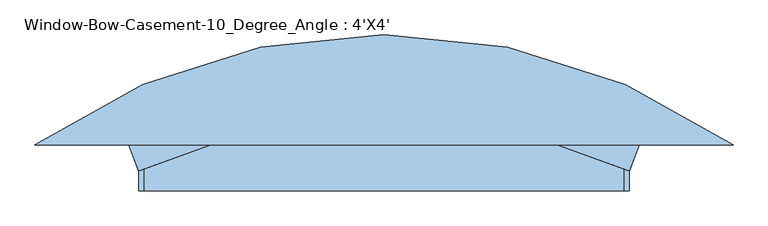
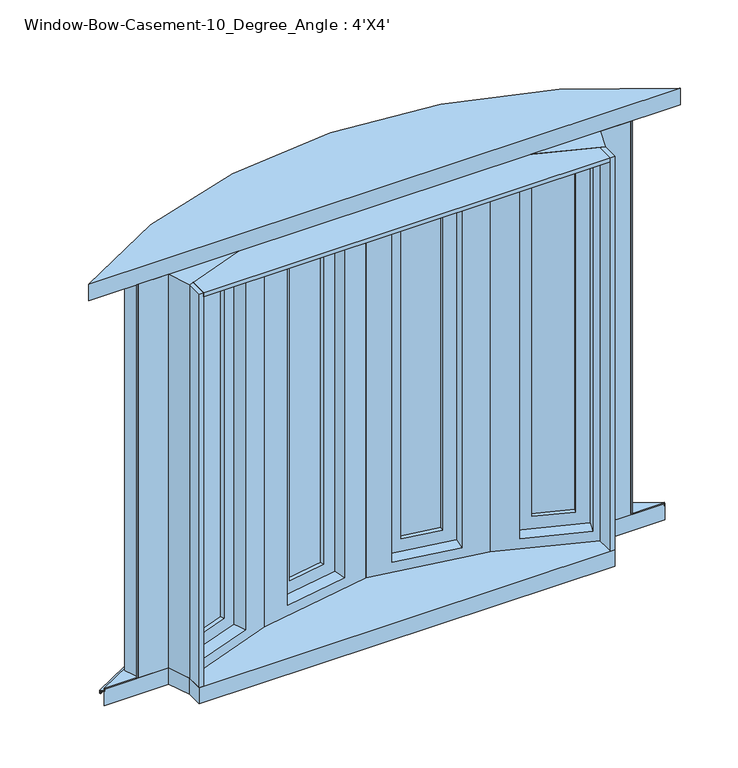
"""IFC4 building model written with IfcOpenShell, lengths in millimetres: window geometry, Window-Bow-Casement-10_Degree_Angle : 4'X4'."""

from ifc_helpers import new_model, si_unit, point, frame, frame_2d, origin, place, context, project, spatial, polyline, circle_curve, trimmed, segment, composite_curve, outline, extrude, faceted_brep, source, transform, mapped, element, save
from ifc_brep_helpers import plane_surface, cylinder_surface, revolved_surface, advanced_brep


def window_bow_casement_10_degree_angle_4_x4_a8433a54(model_context):
    return source(origin(), model_context, "Body", "SolidModel", [
        advanced_brep(
        [(-820.9076978, 57.15, 663.1486341), (-820.9076978, 57.15, 660.4), (-728.4786409, 57.15, 660.4), (-728.4786409, 57.15, 663.1486341), (820.9076978, 57.15, 660.4), (820.9076978, 57.15, 663.1486341), (728.4786409, 57.15, 663.1486341), (728.4786409, 57.15, 660.4), (-820.9076978, 57.15, 653.0697935), (-821.7069058, 58.2958078, 663.1486341), (-821.7069058, 58.2958078, 654.4483503), (-828.9724329, 68.7122427, 652.2089977), (-828.9724329, 68.7122427, 643.2668038), (-826.7055885, 65.4623151, 643.2668038), (-826.7055885, 65.4623151, 644.7270038), (-828.0569765, 67.399772, 644.7270038), (-828.0569765, 67.399772, 650.8662705), (820.9076978, 57.15, 653.0697935), (828.0569765, 67.399772, 650.8662705), (828.0569765, 67.399772, 644.7270038), (826.7055885, 65.4623151, 644.7270038), (826.7055885, 65.4623151, 643.2668038), (828.9724329, 68.7122427, 643.2668038), (828.9724329, 68.7122427, 652.2089977), (821.7069058, 58.2958078, 654.4483503), (821.7069058, 58.2958078, 663.1486341)],
        [
            (0, 1),
            (1, 2),
            (2, 3),
            (3, 0),
            (4, 5),
            (5, 6),
            (6, 7),
            (7, 4),
            (8, 1),
            (0, 9),
            (9, 10),
            (10, 11),
            (11, 12),
            (12, 13),
            (13, 14),
            (14, 15),
            (15, 16),
            (16, 8),
            (17, 18),
            (18, 19),
            (19, 20),
            (20, 21),
            (21, 22),
            (22, 23),
            (23, 24),
            (24, 25),
            (25, 5),
            (4, 17),
            (8, 17, circle_curve(frame((0.0, -1119.7682794, 653.0697935), z_axis=(0.0, 0.0, -1.0), x_axis=(-0.5720887452257101, 0.8201917261141279, 0.0)), 1434.9306899)),
            (4, 1, circle_curve(frame((0.0, -1119.7682794, 660.4), z_axis=(0.0, 0.0, 1.0), x_axis=(-0.5720887452257101, 0.8201917261141279, 0.0)), 1434.9306899)),
            (7, 2, circle_curve(frame((0.0, -1119.7682794, 660.4), z_axis=(0.0, 0.0, 1.0), x_axis=(-0.5720887452257101, 0.8201917261141279, 0.0)), 1384.1306899)),
            (6, 3, circle_curve(frame((0.0, -1119.7682794, 663.1486341), z_axis=(0.0, 0.0, 1.0), x_axis=(-0.5720887452257101, 0.8201917261141279, 0.0)), 1384.1306899)),
            (25, 9, circle_curve(frame((0.0, -1119.7682794, 663.1486341), z_axis=(0.0, 0.0, 1.0), x_axis=(-0.5720887452257101, 0.8201917261141279, 0.0)), 1436.3276898)),
            (24, 10, circle_curve(frame((0.0, -1119.7682794, 654.4483503), z_axis=(0.0, 0.0, 1.0), x_axis=(-0.5720887452257101, 0.8201917261141279, 0.0)), 1436.3276898)),
            (23, 11, circle_curve(frame((0.0, -1119.7682794, 652.2089977), z_axis=(0.0, 0.0, 1.0), x_axis=(-0.5720887452257101, 0.8201917261141279, 0.0)), 1449.0276898)),
            (22, 12, circle_curve(frame((0.0, -1119.7682794, 643.2668038), z_axis=(0.0, 0.0, 1.0), x_axis=(-0.5720887452257101, 0.8201917261141279, 0.0)), 1449.0276898)),
            (21, 13, circle_curve(frame((0.0, -1119.7682794, 643.2668038), z_axis=(0.0, 0.0, 1.0), x_axis=(-0.5720887452257101, 0.8201917261141279, 0.0)), 1445.0652899)),
            (20, 14, circle_curve(frame((0.0, -1119.7682794, 644.7270038), z_axis=(0.0, 0.0, 1.0), x_axis=(-0.5720887452257101, 0.8201917261141279, 0.0)), 1445.0652899)),
            (19, 15, circle_curve(frame((0.0, -1119.7682794, 644.7270038), z_axis=(0.0, 0.0, 1.0), x_axis=(-0.5720887452257101, 0.8201917261141279, 0.0)), 1447.4274899)),
            (18, 16, circle_curve(frame((0.0, -1119.7682794, 650.8662705), z_axis=(0.0, 0.0, 1.0), x_axis=(-0.5720887452257101, 0.8201917261141279, 0.0)), 1447.4274899)),
        ],
        [
            plane_surface(frame((903.8545728, 57.15, 1270.0), z_axis=(0.0, -1.0, 0.0), x_axis=(0.0, 0.0, -1.0))),
            plane_surface(frame((-820.9076978, 57.15, 660.4), z_axis=(-0.8201917261141279, -0.5720887452257101, 0.0), x_axis=(0.0, 0.0, 1.0))),
            plane_surface(frame((820.9076978, 57.15, 660.4), z_axis=(0.8201917261141279, -0.5720887452257102, 0.0), x_axis=(0.0, 0.0, 1.0))),
            revolved_surface(polyline([(-820.9076978707535, 57.15000000321743, 653.0697935), (-820.9076978707535, 57.15000000321743, 660.4)]), (0.0, -1119.7682794, 660.4), (0.0, 0.0, -1.0)),
            plane_surface(frame((0.0, -1119.7682794, 660.4), z_axis=(0.0, 0.0, -1.0), x_axis=(-0.5720887452257101, 0.8201917261141279, 0.0))),
            revolved_surface(polyline([(-791.8455896132875, 15.484260316619839, 660.4), (-791.8455896132875, 15.484260316619839, 663.1486341)]), (0.0, -1119.7682794, 660.4), (0.0, 0.0, -1.0)),
            plane_surface(frame((0.0, -1119.7682794, 663.1486341), z_axis=(0.0, 0.0, 1.0), x_axis=(-0.5720887452257101, 0.8201917261141279, 0.0))),
            cylinder_surface(frame((0.0, -1119.7682794, 660.4), z_axis=(0.0, 0.0, -1.0), x_axis=(-0.5720887452257101, 0.8201917261141279, 0.0)), 1436.3276898),
            revolved_surface(polyline([(-821.7069058, 58.2958078, 654.4483503), (-828.9724329, 68.7122427, 652.2089977)]), (0.0, -1119.7682794, 660.4), (0.0, 0.0, -1.0)),
            cylinder_surface(frame((0.0, -1119.7682794, 660.4), z_axis=(0.0, 0.0, -1.0), x_axis=(-0.5720887452257101, 0.8201917261141279, 0.0)), 1449.0276898),
            plane_surface(frame((0.0, -1119.7682794, 643.2668038), z_axis=(0.0, 0.0, -1.0), x_axis=(-0.5720887452257101, 0.8201917261141279, 0.0))),
            revolved_surface(polyline([(-826.7055884681179, 65.46231507069365, 643.2668038), (-826.7055884681179, 65.46231507069365, 644.7270038)]), (0.0, -1119.7682794, 660.4), (0.0, 0.0, -1.0)),
            plane_surface(frame((0.0, -1119.7682794, 644.7270038), z_axis=(0.0, 0.0, 1.0), x_axis=(-0.5720887452257101, 0.8201917261141279, 0.0))),
            revolved_surface(polyline([(-828.0569765020902, 67.3997719661204, 644.7270038), (-828.0569765020902, 67.3997719661204, 650.8662705)]), (0.0, -1119.7682794, 660.4), (0.0, 0.0, -1.0)),
            revolved_surface(polyline([(-828.0569765, 67.399772, 650.8662705), (-820.9076978, 57.15, 653.0697935)]), (0.0, -1119.7682794, 660.4), (0.0, 0.0, -1.0)),
        ],
        [
            (0, [[1, 2, 3, 4]]),
            (0, [[5, 6, 7, 8]]),
            (1, [[9, -1, 10, 11, 12, 13, 14, 15, 16, 17, 18]]),
            (2, [[19, 20, 21, 22, 23, 24, 25, 26, 27, -5, 28]]),
            (3, [[-9, 29, -28, 30]]),
            (4, [[-30, -8, 31, -2]]),
            (5, [[-31, -7, 32, -3]]),
            (6, [[33, -10, -4, -32, -6, -27]]),
            (7, [[-11, -33, -26, 34]]),
            (8, [[-12, -34, -25, 35]]),
            (9, [[-13, -35, -24, 36]]),
            (10, [[-14, -36, -23, 37]]),
            (11, [[-15, -37, -22, 38]]),
            (12, [[-16, -38, -21, 39]]),
            (13, [[-17, -39, -20, 40]]),
            (14, [[-18, -40, -19, -29]]),
        ],
    ),
        extrude(outline(polyline([(-692.8458946, 68.0091396), (-722.6811353, 57.15), (-737.8839307, 98.919337), (-708.04869, 109.7784765), (-692.8458946, 68.0091396)])), frame((0.0, 0.0, 663.1486341), z_axis=(0.0, 0.0, 1.0), x_axis=(1.0, 0.0, 0.0)), (0.0, 0.0, 1.0), 1216.4513659),
        extrude(outline(polyline([(692.8458946, 68.0091396), (708.04869, 109.7784765), (737.8839307, 98.919337), (722.6811353, 57.15), (692.8458946, 68.0091396)])), frame((0.0, 0.0, 663.1486341), z_axis=(0.0, 0.0, 1.0), x_axis=(1.0, 0.0, 0.0)), (0.0, 0.0, 1.0), 1216.4513659),
        faceted_brep([(0.0, 151.3819163, 1879.6), (330.4505105, 93.1145755, 1879.6), (356.846972, 191.6275109, 1879.6), (0.0, 254.5492601, 1879.6), (280.5494558, 140.6012317, 1866.9), (57.0219627, 180.0151597, 1866.9), (68.048622, 242.550452, 1866.9), (291.5761151, 203.1365241, 1866.9), (255.1728726, 106.3880541, 1847.85), (69.1665548, 139.1859865, 1847.85), (75.7825504, 176.7071619, 1847.85), (261.7888681, 143.9092295, 1847.85), (57.0219627, 180.0151597, 673.1), (68.048622, 242.550452, 673.1), (69.1665548, 139.1859865, 692.15), (75.7825504, 176.7071619, 692.15), (0.0, 254.5492601, 660.4), (356.846972, 191.6275109, 660.4), (330.4505105, 93.1145755, 660.4), (0.0, 151.3819163, 660.4), (280.5494558, 140.6012317, 673.1), (291.5761151, 203.1365241, 673.1), (255.1728726, 106.3880541, 692.15), (261.7888681, 143.9092295, 692.15)], [[[0, 1, 2, 3]], [[4, 5, 6, 7]], [[8, 9, 10, 11]], [[5, 12, 13, 6]], [[9, 14, 15, 10]], [[16, 17, 18, 19]], [[12, 20, 21, 13]], [[14, 22, 23, 15]], [[2, 17, 16, 3], [6, 13, 21, 7]], [[7, 21, 20, 4]], [[4, 20, 12, 5], [10, 15, 23, 11]], [[11, 23, 22, 8]], [[18, 1, 0, 19], [8, 22, 14, 9]], [[3, 16, 19, 0]], [[1, 18, 17, 2]]]),
        extrude(outline(polyline([(229.7810224, 181.7928712), (228.6783565, 175.539342), (117.7143895, 195.1052833), (118.8170554, 201.3588125), (229.7810224, 181.7928712)])), frame((0.0, 0.0, 730.25), z_axis=(0.0, 0.0, 1.0), x_axis=(1.0, 0.0, 0.0)), (0.0, 0.0, 1.0), 1079.5),
        extrude(outline(polyline([(227.5756905, 169.2858128), (226.4730246, 163.0322836), (115.5090576, 182.5982248), (116.6117235, 188.8517541), (227.5756905, 169.2858128)])), frame((0.0, 0.0, 730.25), z_axis=(0.0, 0.0, 1.0), x_axis=(1.0, 0.0, 0.0)), (0.0, 0.0, 1.0), 1079.5),
        extrude(outline(polyline([(1136.65, 57.1499999), (1136.65, -169.8257651), (-57.15, -169.8257651), (-57.15, 57.1499999), (1136.65, 57.1499999)]), holes=[polyline([(1079.5, -112.6757651), (1079.5, 0.0), (0.0, 0.0), (0.0, -112.6757651), (1079.5, -112.6757651)])]), frame((224.2676928, 150.5252251, 730.25), z_axis=(0.17364817766693014, 0.9848077530122081, 0.0), x_axis=(0.0, 0.0, 1.0)), (0.0, 0.0, 1.0), 44.45),
        faceted_brep([(0.0, 151.3819163, 1879.6), (0.0, 254.5492601, 1879.6), (-356.846972, 191.6275109, 1879.6), (-330.4505105, 93.1145755, 1879.6), (-280.5494558, 140.6012317, 1866.9), (-291.5761151, 203.1365241, 1866.9), (-68.048622, 242.550452, 1866.9), (-57.0219627, 180.0151597, 1866.9), (-255.1728726, 106.3880541, 1847.85), (-261.7888681, 143.9092295, 1847.85), (-75.7825504, 176.7071619, 1847.85), (-69.1665548, 139.1859865, 1847.85), (-68.048622, 242.550452, 673.1), (-57.0219627, 180.0151597, 673.1), (-75.7825504, 176.7071619, 692.15), (-69.1665548, 139.1859865, 692.15), (0.0, 254.5492601, 660.4), (0.0, 151.3819163, 660.4), (-330.4505105, 93.1145755, 660.4), (-356.846972, 191.6275109, 660.4), (-291.5761151, 203.1365241, 673.1), (-280.5494558, 140.6012317, 673.1), (-261.7888681, 143.9092295, 692.15), (-255.1728726, 106.3880541, 692.15)], [[[0, 1, 2, 3]], [[4, 5, 6, 7]], [[8, 9, 10, 11]], [[7, 6, 12, 13]], [[11, 10, 14, 15]], [[16, 17, 18, 19]], [[13, 12, 20, 21]], [[15, 14, 22, 23]], [[2, 1, 16, 19], [6, 5, 20, 12]], [[5, 4, 21, 20]], [[4, 7, 13, 21], [10, 9, 22, 14]], [[9, 8, 23, 22]], [[18, 17, 0, 3], [8, 11, 15, 23]], [[1, 0, 17, 16]], [[3, 2, 19, 18]]]),
        extrude(outline(polyline([(-229.7810224, 181.7928712), (-118.8170554, 201.3588125), (-117.7143895, 195.1052833), (-228.6783565, 175.539342), (-229.7810224, 181.7928712)])), frame((0.0, 0.0, 730.25), z_axis=(0.0, 0.0, 1.0), x_axis=(1.0, 0.0, 0.0)), (0.0, 0.0, 1.0), 1079.5),
        extrude(outline(polyline([(-227.5756905, 169.2858128), (-116.6117235, 188.8517541), (-115.5090576, 182.5982248), (-226.4730246, 163.0322836), (-227.5756905, 169.2858128)])), frame((0.0, 0.0, 730.25), z_axis=(0.0, 0.0, 1.0), x_axis=(1.0, 0.0, 0.0)), (0.0, 0.0, 1.0), 1079.5),
        extrude(outline(polyline([(1136.65, -57.1499999), (-57.15, -57.1499999), (-57.15, 169.8257651), (1136.65, 169.8257651), (1136.65, -57.1499999)]), holes=[polyline([(1079.5, 112.6757651), (0.0, 112.6757651), (0.0, 0.0), (1079.5, 0.0), (1079.5, 112.6757651)])]), frame((-224.2676928, 150.5252251, 730.25), z_axis=(-0.17364817766693014, 0.9848077530122081, 0.0), x_axis=(0.0, 0.0, 1.0)), (0.0, 0.0, 1.0), 44.45),
        faceted_brep([(330.4505105, 93.1145755, 1879.6), (609.6, -8.4875296, 1879.6), (633.490107, 57.15, 1879.6), (726.3208967, 57.15, 1879.6), (356.846972, 191.6275109, 1879.6), (610.6968712, 31.6584151, 1866.9), (397.4094197, 109.2886988, 1866.9), (419.1276988, 168.9591802, 1866.9), (632.4151503, 91.3288965, 1866.9), (579.7647593, 2.37161, 1847.85), (402.2795966, 66.9709262, 1847.85), (415.3105641, 102.7732151, 1847.85), (592.7957267, 38.1738988, 1847.85), (397.4094197, 109.2886988, 673.1), (419.1276988, 168.9591802, 673.1), (402.2795966, 66.9709262, 692.15), (415.3105641, 102.7732151, 692.15), (356.846972, 191.6275109, 660.4), (726.3208967, 57.15, 660.4), (633.490107, 57.15, 660.4), (609.6, -8.4875296, 660.4), (330.4505105, 93.1145755, 660.4), (610.6968712, 31.6584151, 673.1), (632.4151503, 91.3288965, 673.1), (579.7647593, 2.37161, 692.15), (592.7957267, 38.1738988, 692.15)], [[[0, 1, 2, 3, 4]], [[5, 6, 7, 8]], [[9, 10, 11, 12]], [[6, 13, 14, 7]], [[10, 15, 16, 11]], [[17, 18, 19, 20, 21]], [[13, 22, 23, 14]], [[15, 24, 25, 16]], [[20, 19, 2, 1]], [[3, 18, 17, 4], [7, 14, 23, 8]], [[8, 23, 22, 5]], [[5, 22, 13, 6], [11, 16, 25, 12]], [[12, 25, 24, 9]], [[1, 0, 21, 20], [9, 24, 15, 10]], [[2, 19, 18, 3]], [[4, 17, 21, 0]]]),
        extrude(outline(polyline([(567.8525774, 81.040107), (565.6807495, 75.0730589), (459.8001646, 113.6104402), (461.9719925, 119.5774883), (567.8525774, 81.040107)])), frame((0.0, 0.0, 730.25), z_axis=(0.0, 0.0, 1.0), x_axis=(1.0, 0.0, 0.0)), (0.0, 0.0, 1.0), 1079.5),
        extrude(outline(polyline([(563.5089216, 69.1060107), (561.3370937, 63.1389626), (455.4565088, 101.6763439), (457.6283367, 107.643392), (563.5089216, 69.1060107)])), frame((0.0, 0.0, 730.25), z_axis=(0.0, 0.0, 1.0), x_axis=(1.0, 0.0, 0.0)), (0.0, 0.0, 1.0), 1079.5),
        extrude(outline(polyline([(1136.65, 57.15), (1136.65, -169.825765), (-57.15, -169.825765), (-57.15, 57.15), (1136.65, 57.15)]), holes=[polyline([(1079.5, -112.6757651), (1079.5, 0.0), (0.0, 0.0), (0.0, -112.6757651), (1079.5, -112.6757651)])]), frame((556.9934379, 51.2048663, 730.25), z_axis=(0.3420201433256678, 0.9396926207859088, 0.0), x_axis=(0.0, 0.0, 1.0)), (0.0, 0.0, 1.0), 44.45),
        faceted_brep([(-330.4505105, 93.1145755, 1879.6), (-356.846972, 191.6275109, 1879.6), (-726.3208967, 57.15, 1879.6), (-633.490107, 57.15, 1879.6), (-609.6, -8.4875296, 1879.6), (-610.6968712, 31.6584151, 1866.9), (-632.4151503, 91.3288965, 1866.9), (-419.1276988, 168.9591802, 1866.9), (-397.4094197, 109.2886988, 1866.9), (-579.7647593, 2.37161, 1847.85), (-592.7957267, 38.1738988, 1847.85), (-415.3105641, 102.7732151, 1847.85), (-402.2795966, 66.9709262, 1847.85), (-419.1276988, 168.9591802, 673.1), (-397.4094197, 109.2886988, 673.1), (-415.3105641, 102.7732151, 692.15), (-402.2795966, 66.9709262, 692.15), (-356.846972, 191.6275109, 660.4), (-330.4505105, 93.1145755, 660.4), (-609.6, -8.4875296, 660.4), (-633.490107, 57.15, 660.4), (-726.3208967, 57.15, 660.4), (-632.4151503, 91.3288965, 673.1), (-610.6968712, 31.6584151, 673.1), (-592.7957267, 38.1738988, 692.15), (-579.7647593, 2.37161, 692.15)], [[[0, 1, 2, 3, 4]], [[5, 6, 7, 8]], [[9, 10, 11, 12]], [[8, 7, 13, 14]], [[12, 11, 15, 16]], [[17, 18, 19, 20, 21]], [[14, 13, 22, 23]], [[16, 15, 24, 25]], [[19, 4, 3, 20]], [[2, 1, 17, 21], [7, 6, 22, 13]], [[6, 5, 23, 22]], [[5, 8, 14, 23], [11, 10, 24, 15]], [[10, 9, 25, 24]], [[4, 19, 18, 0], [9, 12, 16, 25]], [[3, 2, 21, 20]], [[1, 0, 18, 17]]]),
        extrude(outline(polyline([(-567.8525774, 81.040107), (-461.9719925, 119.5774883), (-459.8001646, 113.6104402), (-565.6807495, 75.0730589), (-567.8525774, 81.040107)])), frame((0.0, 0.0, 730.25), z_axis=(0.0, 0.0, 1.0), x_axis=(1.0, 0.0, 0.0)), (0.0, 0.0, 1.0), 1079.5),
        extrude(outline(polyline([(-563.5089216, 69.1060107), (-457.6283367, 107.643392), (-455.4565088, 101.6763439), (-561.3370937, 63.1389626), (-563.5089216, 69.1060107)])), frame((0.0, 0.0, 730.25), z_axis=(0.0, 0.0, 1.0), x_axis=(1.0, 0.0, 0.0)), (0.0, 0.0, 1.0), 1079.5),
        extrude(outline(polyline([(1136.65, -57.15), (-57.15, -57.15), (-57.15, 169.825765), (1136.65, 169.825765), (1136.65, -57.15)]), holes=[polyline([(1079.5, 112.6757651), (0.0, 112.6757651), (0.0, 0.0), (1079.5, 0.0), (1079.5, 112.6757651)])]), frame((-556.9934379, 51.2048663, 730.25), z_axis=(-0.3420201433256678, 0.9396926207859088, 0.0), x_axis=(0.0, 0.0, 1.0)), (0.0, 0.0, 1.0), 44.45),
        extrude(outline(composite_curve([segment(trimmed(circle_curve(frame_2d((0.0, -1180.3814298)), 1511.1306899), [point((-867.1977411, 57.15))], [point((867.1977411, 57.15))], False, "CARTESIAN"), True, "CONTINUOUS"), segment(polyline([(867.1977411, 57.15), (-867.1977411, 57.15)]), True, "CONTINUOUS")], self_intersect=False)), frame((0.0, 0.0, 1879.6), z_axis=(0.0, 0.0, 1.0), x_axis=(1.0, 0.0, 0.0)), (0.0, 0.0, 1.0), 50.8),
        extrude(outline(polyline([(-609.6, -57.15), (-609.6, -8.4875296), (-596.9, -3.8651076), (-596.9, -57.15), (-609.6, -57.15)])), frame((0.0, 0.0, 660.4), z_axis=(0.0, 0.0, 1.0), x_axis=(1.0, 0.0, 0.0)), (0.0, 0.0, 1.0), 1219.2),
        extrude(outline(polyline([(609.6, -57.15), (596.9, -57.15), (596.9, -3.8651076), (609.6, -8.4875296), (609.6, -57.15)])), frame((0.0, 0.0, 660.4), z_axis=(0.0, 0.0, 1.0), x_axis=(1.0, 0.0, 0.0)), (0.0, 0.0, 1.0), 1219.2),
        extrude(outline(polyline([(-330.4505105, 93.1145755), (0.0, 151.3819163), (330.4505105, 93.1145755), (596.9, -3.8651076), (596.9, -57.15), (-596.9, -57.15), (-596.9, -3.8651076), (-330.4505105, 93.1145755)])), frame((0.0, 0.0, 1866.9), z_axis=(0.0, 0.0, 1.0), x_axis=(1.0, 0.0, 0.0)), (0.0, 0.0, 1.0), 12.7),
        extrude(outline(composite_curve([segment(trimmed(circle_curve(frame_2d((0.0, -1180.3814298)), 1485.7306899), [point((-822.1384574, 57.15))], [point((822.1384574, 57.15))], False, "CARTESIAN"), True, "CONTINUOUS"), segment(polyline([(822.1384574, 57.15), (633.490107, 57.15), (609.6, -8.4875296), (609.6, -57.15), (-609.6, -57.15), (-609.6, -8.4875296), (-633.490107, 57.15), (-822.1384574, 57.15)]), True, "CONTINUOUS")], self_intersect=False)), frame((0.0, 0.0, 609.6), z_axis=(0.0, 0.0, 1.0), x_axis=(1.0, 0.0, 0.0)), (0.0, 0.0, 1.0), 50.8),
    ])


if __name__ == "__main__":
    model = new_model("IFC4")
    model_context = context("Model", 3, world=origin())
    ifc_project = project(units=[si_unit("LENGTHUNIT", "METRE", prefix="MILLI")], contexts=[model_context])
    site = spatial("IfcSite", under=ifc_project)
    building = spatial("IfcBuilding", under=site)
    placement = place(None, origin())
    window_bow_casement_10_degree_angle_4_x4_shape = window_bow_casement_10_degree_angle_4_x4_a8433a54(model_context)
    element("IfcWindow", 1, ObjectType="Window-Bow-Casement-10_Degree_Angle : 4'X4'", at=placement, inside=building, context=model_context, shape_type="MappedRepresentation", body=[
        mapped(window_bow_casement_10_degree_angle_4_x4_shape, transform((0.0, 0.0, 0.0), x_axis=(1.0, 0.0, 0.0), y_axis=(0.0, 1.0, 0.0), z_axis=(0.0, 0.0, 1.0))),
    ])
    save(model, "model.ifc")

# Revit data of these elements
# Type "Window-Bow-Casement-10_Degree_Angle : 4'X4'"
#   Type Mark = "27"
#   Fire Rating = "0.5h"
#   Assembly Code = "B2020100"
#   Analytic Construction = "Double glazing - domestic"
#   Width = 4' - 0"
#   Visual Light Transmittance = 0.81
#   Thermal Resistance (R) = 1.8146 (h·ft²·°F)/BTU
#   Solar Heat Gain Coefficient = 0.76
#   Rough Width = 4' - 0 1/2"
#   Rough Height = 4' - 0 1/2"
#   Radius 3 = 4' - 11.49333"
#   Radius 2 = 4' - 10.49333"
#   Radius 1 = 4' - 8.49333"
#   Length 7 = 4' - 9.19062"
#   Length 6 = 0' - 1.41593"
#   Length 5 = 1' - 1.00986"
#   Length 2 = 0' - 2.58415"
#   Depth 2 = 0' - 6.3557"
#   Length 4 = 0' - 1.03923"
#   Length 3 = 0' - 0.32476"
#   Length 1 = 0' - 10.27567"
#   Wall Thickness [instance default] = 0' - 6"
#   Trim Width = 4' - 4.64952"
#   Trim Height = 4' - 0"
#   Height 1 = 4' - 2"
#   Height = 4' - 0"
#   Heat Transfer Coefficient (U) = 0.5511 BTU/(h·ft²·°F)
#   Depth 1 = 0' - 5.29439"
#   Default Sill Height = 2' - 0"
#   Angle 2 = 15.00°
#   Angle 1 = 10.00°
#   Angle = 20.00°
#   Muntin Visibility = yes
#   Interior Trim Visibility [instance default] = yes
#   Exterior Trim Visibility [instance default] = yes
#   Muntin Pattern = Muntin Pattern_2x2 : Muntin Pattern_2x2
#   Interior Trim Material = Wood - Stained
#   Exterior Trim Material = Clad - White
#   Interior Trim = Trim-Window-Interior-Flat : Picture Frame
#   Interior Frame Material = Wood - Stained
#   Glass Panel Material = Glass
#   Exterior Frame Material = Clad - White
#   Wall Closure = (empty or 0)
# Element 1 (IfcWindow, "Window-Bow-Casement-10_Degree_Angle : 4'X4'")
#   Wall Thickness = 0' - 4 1/2"
#   Materials on its faces: "Wood - Stained", "Clad - White", "Glass"
# Materials
#   "Wood - Stained": class "Wood", colour RGB 224 178 126, transparency 0, Cost = 0
#   "Clad - White": class "Wood", colour RGB 242 242 238, transparency 0, Cost = 0
#   "Glass": class "Glass", colour RGB 0 128 192, transparency 0.75, Description = "Soda Lime Glass", Cost = 0
